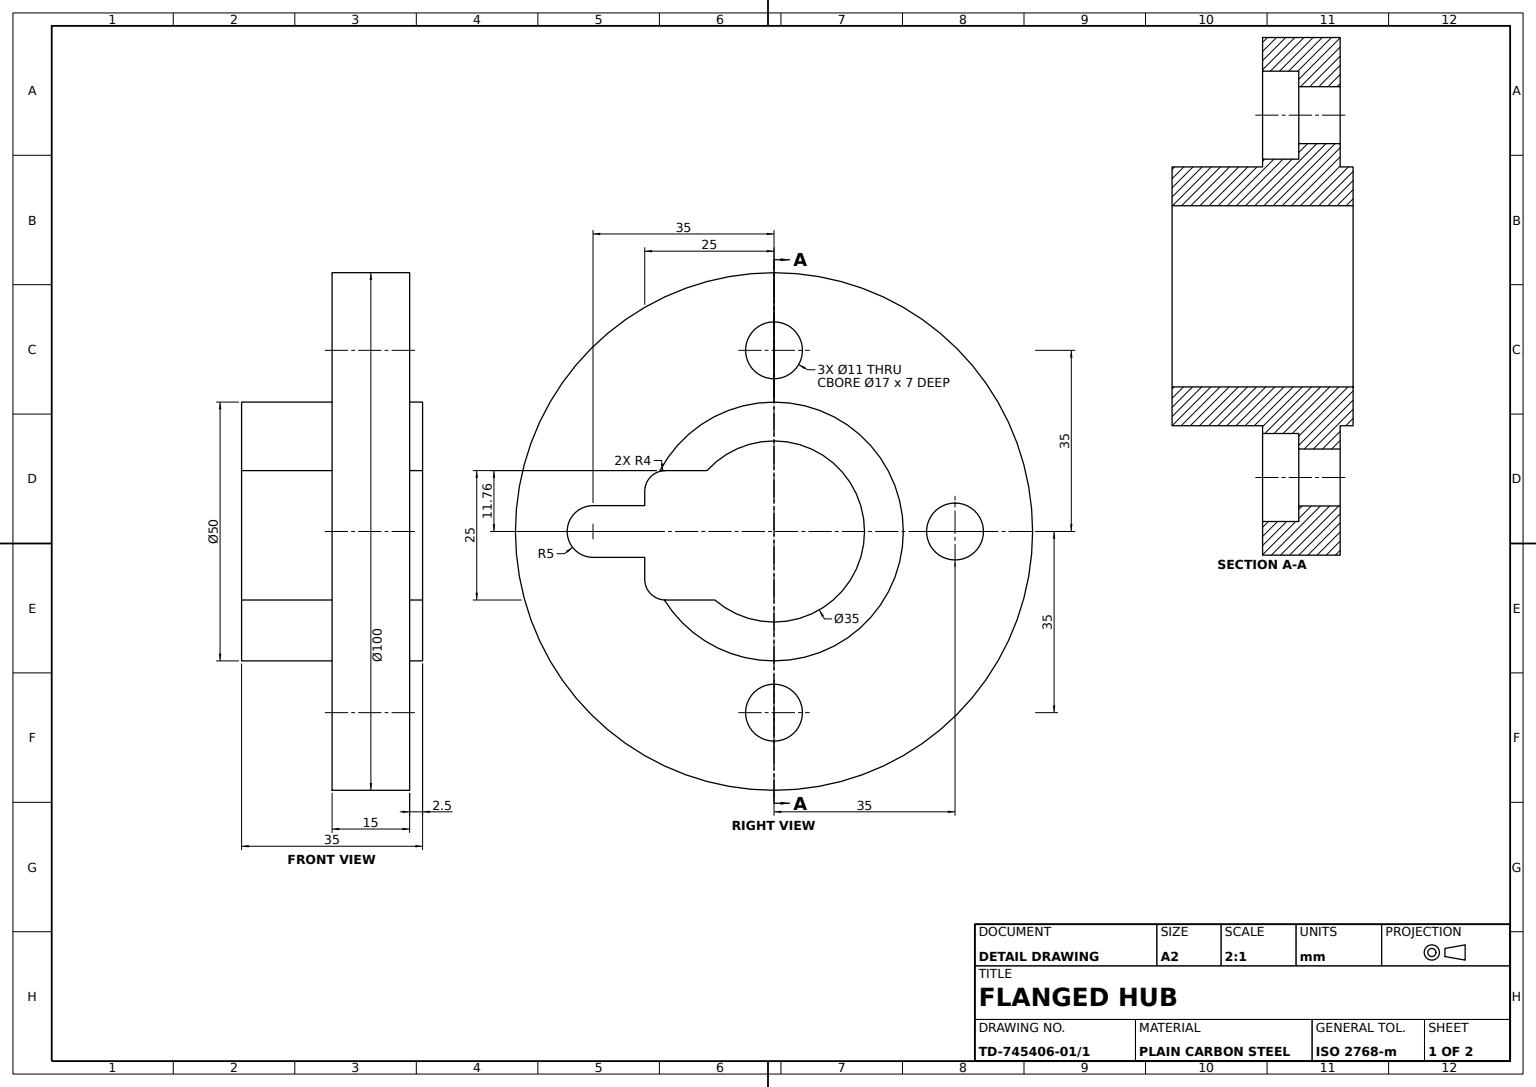
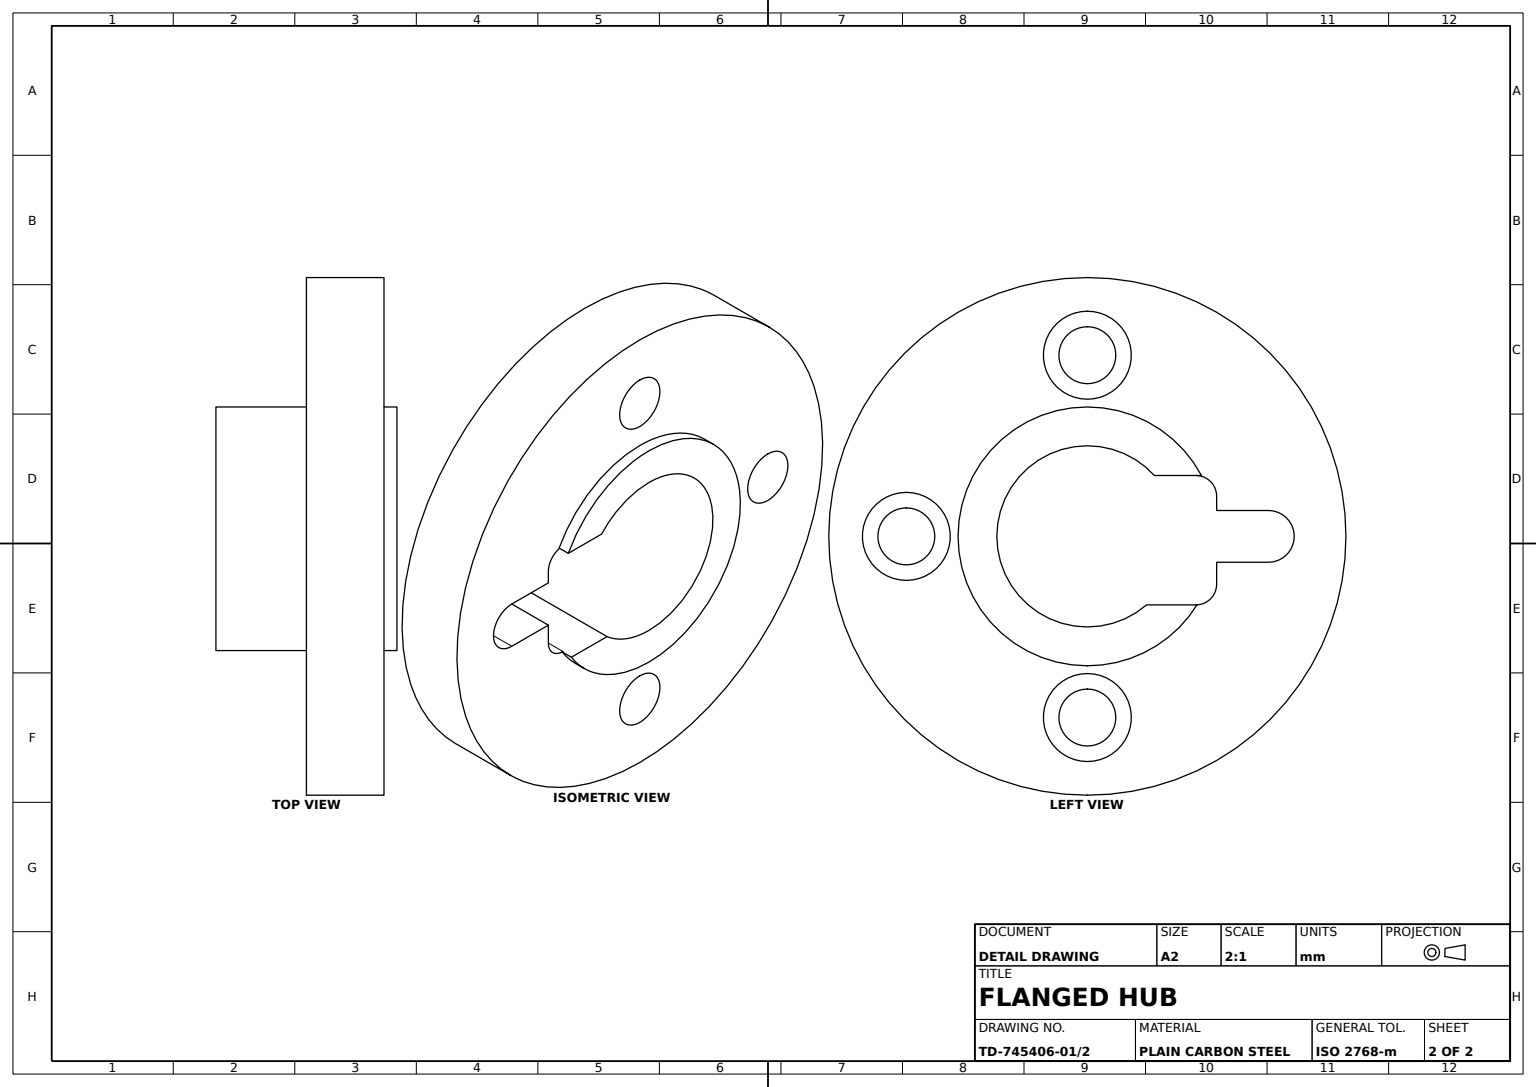
from build123d import *

# Parameters (mm, degrees)
FLANGE_PROFILE_SKETCH_R   = 50
FLANGE_PROFILE_SKETCH_R_2 = 5.5
FLANGE_100_DEPTH          = 7.5
HUB_50_DEPTH              = 17.5
HUB_SLOTS_SKETCH_R        = 8.5
HUB_SLOTS_4X_DEPTH        = 7


with BuildPart() as part:
    # Flange Profile Sketch → Flange Ø100 (new, symmetric)
    with BuildSketch(Plane.XY):
        Circle(FLANGE_PROFILE_SKETCH_R)
        with Locations((-35, 0)):
            Circle(FLANGE_PROFILE_SKETCH_R_2, mode=Mode.SUBTRACT)
        with Locations((35, 0)):
            Circle(FLANGE_PROFILE_SKETCH_R_2, mode=Mode.SUBTRACT)
        with Locations((0, -35)):
            Circle(FLANGE_PROFILE_SKETCH_R_2, mode=Mode.SUBTRACT)
        with BuildLine():
            Line((-11.763017547, 12.956906196), (-11.763017547, 21))
            ThreePointArc((-11.763017547, 21), (-10.591444672, 23.828427125), (-7.763017547, 25))
            Line((-7.763017547, 25), (-5, 25))
            Line((-5, 25), (-5, 35))
            ThreePointArc((-5, 35), (0, 40), (5, 35))
            Line((5, 35), (5, 25))
            Line((5, 25), (9.236982453, 25))
            ThreePointArc((9.236982453, 25), (12.065409578, 23.828427125), (13.236982453, 21))
            Line((13.236982453, 21), (13.236982453, 11.446933893))
            ThreePointArc((13.236982453, 11.446933893), (-1.055057925, -17.468166841), (-11.763017547, 12.956906196))
        make_face(mode=Mode.SUBTRACT)
    extrude(amount=FLANGE_100_DEPTH, both=True)

    # Hub Profile Sketch → Hub Ø50 (add, symmetric)
    with BuildSketch(Plane.XY.offset(7.5)):
        with BuildLine():
            Line((-11.763017547, 12.956906196), (-11.763017547, 22.059723892))
            ThreePointArc((-11.763017547, 22.059723892), (-0.851158679, -24.985506377), (13.236982453, 21.208071472))
            Line((13.236982453, 21.208071472), (13.236982453, 11.446933893))
            ThreePointArc((13.236982453, 11.446933893), (-1.055057925, -17.468166841), (-11.763017547, 12.956906196))
        make_face()
    extrude(amount=HUB_50_DEPTH, both=True)

    # Hub Slots Sketch → Hub Slots 4x (cut)
    with BuildSketch(Plane.XY.offset(7.5)):
        with Locations((-35, 0)):
            Circle(HUB_SLOTS_SKETCH_R)
        with Locations((35, 0)):
            Circle(HUB_SLOTS_SKETCH_R)
        with Locations((0, -35)):
            Circle(HUB_SLOTS_SKETCH_R)
    extrude(amount=-HUB_SLOTS_4X_DEPTH, mode=Mode.SUBTRACT)


solid = part.part
